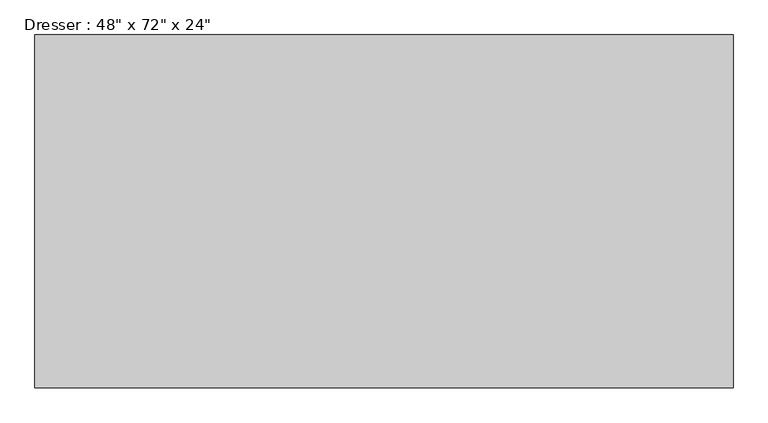
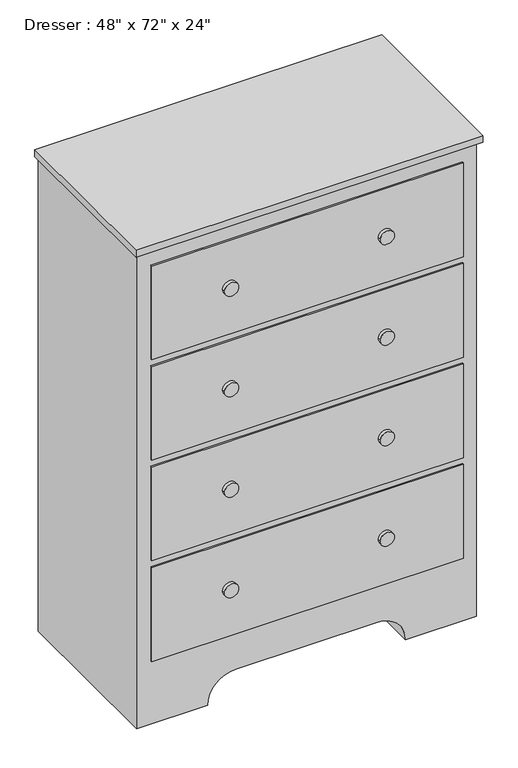
"""IFC4 building model written with IfcOpenShell, lengths in millimetres: furniture geometry."""

from ifc_helpers import new_model, si_unit, point, frame, frame_2d, origin, place, context, project, spatial, polyline, circle_curve, trimmed, segment, composite_curve, outline, extrude, source, transform, mapped, element, save


def furniture_9fa109b2(model_context):
    return source(origin(), model_context, "Body", "SweptSolid", [
        extrude(outline(polyline([(353.1067402, -58.3629541), (353.1067402, -687.0129541), (-891.4932598, -687.0129541), (-891.4932598, -58.3629541), (353.1067402, -58.3629541)])), frame((0.0, 0.0, 1803.4), z_axis=(0.0, 0.0, 1.0), x_axis=(1.0, 0.0, 0.0)), (0.0, 0.0, 1.0), 25.4),
        extrude(outline(composite_curve([segment(polyline([(0.0, 340.4067402), (1803.4, 340.4067402), (1803.4, -878.7932598), (0.0, -878.7932598), (0.0, -624.7932598)]), True, "CONTINUOUS"), segment(trimmed(circle_curve(frame_2d((0.0, -523.1932598)), 101.6), [point((0.0, -624.7932598))], [point((101.6, -523.1932598))], True, "CARTESIAN"), True, "CONTINUOUS"), segment(polyline([(101.6, -523.1932598), (101.6, -15.1932598)]), True, "CONTINUOUS"), segment(trimmed(circle_curve(frame_2d((0.0, -15.1932598)), 101.6), [point((101.6, -15.1932598))], [point((0.0, 86.4067402))], True, "CARTESIAN"), True, "CONTINUOUS"), segment(polyline([(0.0, 86.4067402), (0.0, 340.4067402)]), True, "CONTINUOUS")], self_intersect=False)), frame((0.0, -667.9629541, 0.0), z_axis=(0.0, 1.0, 0.0), x_axis=(0.0, 0.0, 1.0)), (0.0, 0.0, 1.0), 609.6),
        extrude(outline(composite_curve([segment(trimmed(circle_curve(frame_2d((1562.1, 10.2067402)), 25.4), [point((1562.1, -15.1932598))], [point((1562.1, 35.6067402))], False, "CARTESIAN"), True, "CONTINUOUS"), segment(trimmed(circle_curve(frame_2d((1562.1, 10.2067402)), 25.4), [point((1562.1, 35.6067402))], [point((1562.1, -15.1932598))], False, "CARTESIAN"), True, "CONTINUOUS")], self_intersect=False)), frame((0.0, -687.0129541, 0.0), z_axis=(0.0, 1.0, 0.0), x_axis=(0.0, 0.0, 1.0)), (0.0, 0.0, 1.0), 12.7),
        extrude(outline(composite_curve([segment(trimmed(circle_curve(frame_2d((1181.1, 10.2067402)), 25.4), [point((1181.1, -15.1932598))], [point((1181.1, 35.6067402))], False, "CARTESIAN"), True, "CONTINUOUS"), segment(trimmed(circle_curve(frame_2d((1181.1, 10.2067402)), 25.4), [point((1181.1, 35.6067402))], [point((1181.1, -15.1932598))], False, "CARTESIAN"), True, "CONTINUOUS")], self_intersect=False)), frame((0.0, -687.0129541, 0.0), z_axis=(0.0, 1.0, 0.0), x_axis=(0.0, 0.0, 1.0)), (0.0, 0.0, 1.0), 12.7),
        extrude(outline(composite_curve([segment(trimmed(circle_curve(frame_2d((800.1, 10.2067402)), 25.4), [point((800.1, -15.1932598))], [point((800.1, 35.6067402))], False, "CARTESIAN"), True, "CONTINUOUS"), segment(trimmed(circle_curve(frame_2d((800.1, 10.2067402)), 25.4), [point((800.1, 35.6067402))], [point((800.1, -15.1932598))], False, "CARTESIAN"), True, "CONTINUOUS")], self_intersect=False)), frame((0.0, -687.0129541, 0.0), z_axis=(0.0, 1.0, 0.0), x_axis=(0.0, 0.0, 1.0)), (0.0, 0.0, 1.0), 12.7),
        extrude(outline(composite_curve([segment(trimmed(circle_curve(frame_2d((419.1, 10.2067402)), 25.4), [point((419.1, -15.1932598))], [point((419.1, 35.6067402))], False, "CARTESIAN"), True, "CONTINUOUS"), segment(trimmed(circle_curve(frame_2d((419.1, 10.2067402)), 25.4), [point((419.1, 35.6067402))], [point((419.1, -15.1932598))], False, "CARTESIAN"), True, "CONTINUOUS")], self_intersect=False)), frame((0.0, -687.0129541, 0.0), z_axis=(0.0, 1.0, 0.0), x_axis=(0.0, 0.0, 1.0)), (0.0, 0.0, 1.0), 12.7),
        extrude(outline(composite_curve([segment(trimmed(circle_curve(frame_2d((419.1, -548.5932598)), 25.4), [point((419.1, -573.9932598))], [point((419.1, -523.1932598))], False, "CARTESIAN"), True, "CONTINUOUS"), segment(trimmed(circle_curve(frame_2d((419.1, -548.5932598)), 25.4), [point((419.1, -523.1932598))], [point((419.1, -573.9932598))], False, "CARTESIAN"), True, "CONTINUOUS")], self_intersect=False)), frame((0.0, -687.0129541, 0.0), z_axis=(0.0, 1.0, 0.0), x_axis=(0.0, 0.0, 1.0)), (0.0, 0.0, 1.0), 12.7),
        extrude(outline(composite_curve([segment(trimmed(circle_curve(frame_2d((800.1, -548.5932598)), 25.4), [point((800.1, -573.9932598))], [point((800.1, -523.1932598))], False, "CARTESIAN"), True, "CONTINUOUS"), segment(trimmed(circle_curve(frame_2d((800.1, -548.5932598)), 25.4), [point((800.1, -523.1932598))], [point((800.1, -573.9932598))], False, "CARTESIAN"), True, "CONTINUOUS")], self_intersect=False)), frame((0.0, -687.0129541, 0.0), z_axis=(0.0, 1.0, 0.0), x_axis=(0.0, 0.0, 1.0)), (0.0, 0.0, 1.0), 12.7),
        extrude(outline(composite_curve([segment(trimmed(circle_curve(frame_2d((1181.1, -548.5932598)), 25.4), [point((1181.1, -573.9932598))], [point((1181.1, -523.1932598))], False, "CARTESIAN"), True, "CONTINUOUS"), segment(trimmed(circle_curve(frame_2d((1181.1, -548.5932598)), 25.4), [point((1181.1, -523.1932598))], [point((1181.1, -573.9932598))], False, "CARTESIAN"), True, "CONTINUOUS")], self_intersect=False)), frame((0.0, -687.0129541, 0.0), z_axis=(0.0, 1.0, 0.0), x_axis=(0.0, 0.0, 1.0)), (0.0, 0.0, 1.0), 12.7),
        extrude(outline(composite_curve([segment(trimmed(circle_curve(frame_2d((1562.1, -548.5932598)), 25.4), [point((1562.1, -573.9932598))], [point((1562.1, -523.1932598))], False, "CARTESIAN"), True, "CONTINUOUS"), segment(trimmed(circle_curve(frame_2d((1562.1, -548.5932598)), 25.4), [point((1562.1, -523.1932598))], [point((1562.1, -573.9932598))], False, "CARTESIAN"), True, "CONTINUOUS")], self_intersect=False)), frame((0.0, -687.0129541, 0.0), z_axis=(0.0, 1.0, 0.0), x_axis=(0.0, 0.0, 1.0)), (0.0, 0.0, 1.0), 12.7),
        extrude(outline(polyline([(289.6067402, -674.3129541), (-827.9932598, -674.3129541), (-827.9932598, -667.9629541), (289.6067402, -667.9629541), (289.6067402, -674.3129541)])), frame((0.0, 0.0, 1384.3), z_axis=(0.0, 0.0, 1.0), x_axis=(1.0, 0.0, 0.0)), (0.0, 0.0, 1.0), 355.6),
        extrude(outline(polyline([(289.6067402, -674.3129541), (-827.9932598, -674.3129541), (-827.9932598, -667.9629541), (289.6067402, -667.9629541), (289.6067402, -674.3129541)])), frame((0.0, 0.0, 1003.3), z_axis=(0.0, 0.0, 1.0), x_axis=(1.0, 0.0, 0.0)), (0.0, 0.0, 1.0), 355.6),
        extrude(outline(polyline([(289.6067402, -674.3129541), (-827.9932598, -674.3129541), (-827.9932598, -667.9629541), (289.6067402, -667.9629541), (289.6067402, -674.3129541)])), frame((0.0, 0.0, 622.3), z_axis=(0.0, 0.0, 1.0), x_axis=(1.0, 0.0, 0.0)), (0.0, 0.0, 1.0), 355.6),
        extrude(outline(polyline([(289.6067402, -674.3129541), (-827.9932598, -674.3129541), (-827.9932598, -667.9629541), (289.6067402, -667.9629541), (289.6067402, -674.3129541)])), frame((0.0, 0.0, 241.3), z_axis=(0.0, 0.0, 1.0), x_axis=(1.0, 0.0, 0.0)), (0.0, 0.0, 1.0), 355.6),
    ])


if __name__ == "__main__":
    model = new_model("IFC4")
    model_context = context("Model", 3, world=origin())
    ifc_project = project(units=[si_unit("LENGTHUNIT", "METRE", prefix="MILLI")], contexts=[model_context])
    site = spatial("IfcSite", under=ifc_project)
    building = spatial("IfcBuilding", under=site)
    placement = place(None, origin())
    furniture_shape = furniture_9fa109b2(model_context)
    element("IfcFurniture", 1, ObjectType="Dresser : 48\" x 72\" x 24\"", at=placement, inside=building, context=model_context, shape_type="MappedRepresentation", body=[
        mapped(furniture_shape, transform((0.0, 0.0, 0.0), x_axis=(1.0, 0.0, 0.0), y_axis=(0.0, 1.0, 0.0), z_axis=(0.0, 0.0, 1.0))),
    ])
    save(model, "model.ifc")

# Revit data of these elements
# Type "Dresser : 48\" x 72\" x 24\""
#   Assembly Code = "E2020200"
#   Depth = 2' - 0"
#   Height = 6' - 0"
#   Width = 4' - 0"
#   Dresser Material = Laminate - Ivory, Glossy
#   Drawer Material = Laminate, Ivory, Matte
#   Knob Material = Cherry
#   Default Elevation = 0
# Element 1 (IfcFurniture, "Dresser : 48\" x 72\" x 24\"")
#   Materials on its faces: "Laminate, Ivory, Matte", "Cherry", "Laminate - Ivory, Glossy"
# Materials
#   "Laminate - Ivory, Glossy": colour RGB 247 247 239, transparency 0
#   "Laminate, Ivory, Matte": class "Plastic", colour RGB 247 247 239, transparency 0, Description = "Plastic Laminate - Ivory, Matte", Cost = 0
#   "Cherry": class "Wood", colour RGB 226 177 128, transparency 0, Description = "Prunus Serotina", Cost = 0
